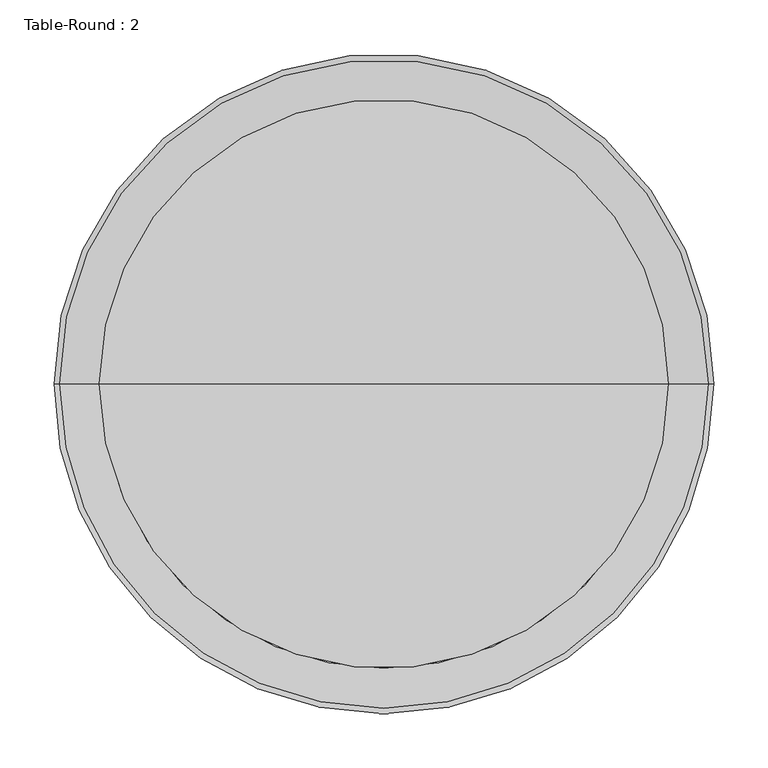
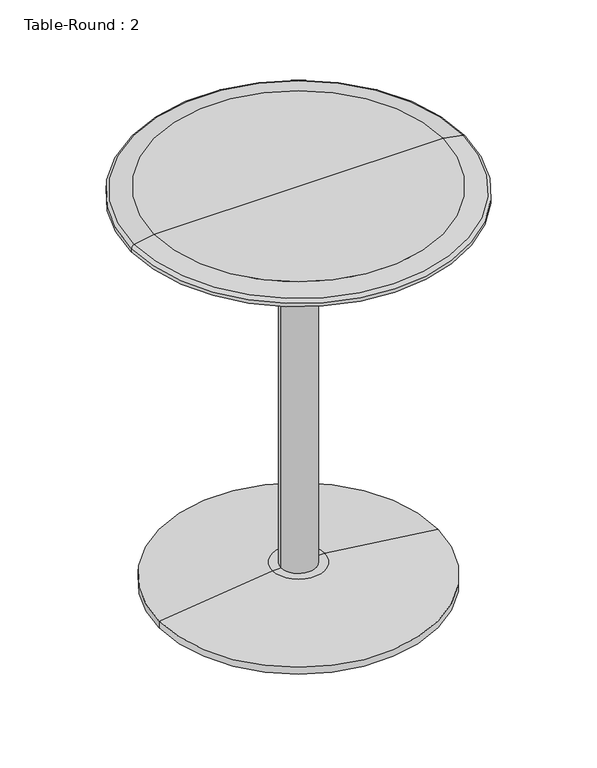
"""IFC4 building model written with IfcOpenShell, lengths in millimetres: furniture geometry, Table-Round : 2."""

from ifc_helpers import new_model, si_unit, point, frame, origin, origin_2d, place, context, project, spatial, polyline, circle_curve, ellipse_curve, trimmed, segment, composite_curve, outline, extrude, source, transform, mapped, element, save
from ifc_brep_helpers import plane_surface, cylinder_surface, revolved_surface, advanced_brep


def table_round_2_a0cc3393(model_context):
    return source(origin(), model_context, "Body", "SolidModel", [
        extrude(outline(composite_curve([segment(trimmed(circle_curve(origin_2d(), 31.75), [point((-31.75, 0.0))], [point((31.75, 0.0))], False, "CARTESIAN"), True, "CONTINUOUS"), segment(trimmed(circle_curve(origin_2d(), 31.75), [point((31.75, 0.0))], [point((-31.75, 0.0))], False, "CARTESIAN"), True, "CONTINUOUS")], self_intersect=False)), frame((0.0, 0.0, 38.1), z_axis=(0.0, 0.0, 1.0), x_axis=(1.0, 0.0, 0.0)), (0.0, 0.0, 1.0), 704.85),
        advanced_brep(
        [(0.0, 0.0, 742.95), (-304.8, 0.0, 742.95), (304.8, 0.0, 742.95), (262.9011364, 0.0, 762.0), (-262.9011364, 0.0, 762.0), (0.0, 0.0, 762.0), (299.5526659, 0.0, 755.5373465), (-299.5526659, 0.0, 755.5373465), (304.8, 0.0, 749.2838172), (-304.8, 0.0, 749.2838172)],
        [
            (0, 1),
            (1, 2, circle_curve(frame((0.0, 0.0, 742.95), z_axis=(0.0, 0.0, -1.0), x_axis=(-1.0, 0.0, 0.0)), 304.8)),
            (2, 0),
            (2, 1, circle_curve(frame((0.0, 0.0, 742.95), z_axis=(0.0, 0.0, -1.0), x_axis=(-1.0, 0.0, 0.0)), 304.8)),
            (3, 4, circle_curve(frame((0.0, 0.0, 762.0), z_axis=(0.0, 0.0, 1.0), x_axis=(-1.0, 0.0, 0.0)), 262.9011364)),
            (4, 5),
            (5, 3),
            (4, 3, circle_curve(frame((0.0, 0.0, 762.0), z_axis=(0.0, 0.0, 1.0), x_axis=(-1.0, 0.0, 0.0)), 262.9011364)),
            (6, 7, circle_curve(frame((0.0, 0.0, 755.5373465), z_axis=(0.0, 0.0, 1.0), x_axis=(-1.0, 0.0, 0.0)), 299.5526659)),
            (7, 4),
            (3, 6),
            (7, 6, circle_curve(frame((0.0, 0.0, 755.5373465), z_axis=(0.0, 0.0, 1.0), x_axis=(-1.0, 0.0, 0.0)), 299.5526659)),
            (8, 9, circle_curve(frame((0.0, 0.0, 749.2838172), z_axis=(0.0, 0.0, 1.0), x_axis=(-1.0, 0.0, 0.0)), 304.8)),
            (9, 7, circle_curve(frame((-298.45, 0.0, 749.2838172), z_axis=(0.0, 1.0, 0.0), x_axis=(1.0, 0.0, 0.0)), 6.35)),
            (6, 8, circle_curve(frame((298.45, 0.0, 749.2838172), z_axis=(0.0, 1.0, 0.0), x_axis=(-1.0, 0.0, 0.0)), 6.35)),
            (9, 8, circle_curve(frame((0.0, 0.0, 749.2838172), z_axis=(0.0, 0.0, 1.0), x_axis=(-1.0, 0.0, 0.0)), 304.8)),
            (1, 9),
            (8, 2),
        ],
        [
            plane_surface(frame((0.0, 0.0, 742.95), z_axis=(0.0, 0.0, -1.0), x_axis=(-1.0, 0.0, 0.0))),
            plane_surface(frame((0.0, 0.0, 762.0), z_axis=(0.0, 0.0, 1.0), x_axis=(-1.0, 0.0, 0.0))),
            revolved_surface(polyline([(-262.9011364, 0.0, 762.0), (-299.5526659, 0.0, 755.5373465)]), (0.0, 0.0, 838.2), (0.0, 0.0, -1.0)),
            revolved_surface(trimmed(ellipse_curve(frame((-298.45, 0.0, 749.2838172), z_axis=(0.0, -1.0, 0.0), x_axis=(1.0, 0.0, 0.0)), 6.35, 6.35), [point((-299.5526659, 0.0, 755.5373465))], [point((-304.8, 0.0, 749.2838172))], True, "CARTESIAN"), (0.0, 0.0, 838.2), (0.0, 0.0, -1.0)),
            cylinder_surface(frame((0.0, 0.0, 838.2), z_axis=(0.0, 0.0, -1.0), x_axis=(-1.0, 0.0, 0.0)), 304.8),
        ],
        [
            (0, [[1, 2, 3]]),
            (0, [[-3, 4, -1]]),
            (1, [[5, 6, 7]]),
            (1, [[8, -7, -6]]),
            (2, [[9, 10, -5, 11]]),
            (2, [[12, -11, -8, -10]]),
            (3, [[13, 14, -9, 15]]),
            (3, [[16, -15, -12, -14]]),
            (4, [[-2, 17, -13, 18]]),
            (4, [[-4, -18, -16, -17]]),
        ],
    ),
        advanced_brep(
        [(0.0, 0.0, 0.0), (-254.0, 0.0, 0.0), (254.0, 0.0, 0.0), (47.625, 0.0, 38.1), (-47.625, 0.0, 38.1), (0.0, 0.0, 38.1), (254.0, 0.0, 12.7), (-254.0, 0.0, 12.7)],
        [
            (0, 1),
            (1, 2, circle_curve(frame((0.0, 0.0, 0.0), z_axis=(0.0, 0.0, -1.0), x_axis=(-1.0, 0.0, 0.0)), 254.0)),
            (2, 0),
            (2, 1, circle_curve(frame((0.0, 0.0, 0.0), z_axis=(0.0, 0.0, -1.0), x_axis=(-1.0, 0.0, 0.0)), 254.0)),
            (3, 4, circle_curve(frame((0.0, 0.0, 38.1), z_axis=(0.0, 0.0, 1.0), x_axis=(-1.0, 0.0, 0.0)), 47.625)),
            (4, 5),
            (5, 3),
            (4, 3, circle_curve(frame((0.0, 0.0, 38.1), z_axis=(0.0, 0.0, 1.0), x_axis=(-1.0, 0.0, 0.0)), 47.625)),
            (6, 7, circle_curve(frame((0.0, 0.0, 12.7), z_axis=(0.0, 0.0, 1.0), x_axis=(-1.0, 0.0, 0.0)), 254.0)),
            (7, 4),
            (3, 6),
            (7, 6, circle_curve(frame((0.0, 0.0, 12.7), z_axis=(0.0, 0.0, 1.0), x_axis=(-1.0, 0.0, 0.0)), 254.0)),
            (1, 7),
            (6, 2),
        ],
        [
            plane_surface(frame((0.0, 0.0, 0.0), z_axis=(0.0, 0.0, -1.0), x_axis=(-1.0, 0.0, 0.0))),
            plane_surface(frame((0.0, 0.0, 38.1), z_axis=(0.0, 0.0, 1.0), x_axis=(-1.0, 0.0, 0.0))),
            revolved_surface(polyline([(-47.625, 0.0, 38.1), (-254.0, 0.0, 12.7)]), (0.0, 0.0, 215.9), (0.0, 0.0, -1.0)),
            cylinder_surface(frame((0.0, 0.0, 215.9), z_axis=(0.0, 0.0, -1.0), x_axis=(-1.0, 0.0, 0.0)), 254.0),
        ],
        [
            (0, [[1, 2, 3]]),
            (0, [[-3, 4, -1]]),
            (1, [[5, 6, 7]]),
            (1, [[8, -7, -6]]),
            (2, [[9, 10, -5, 11]]),
            (2, [[12, -11, -8, -10]]),
            (3, [[-2, 13, -9, 14]]),
            (3, [[-4, -14, -12, -13]]),
        ],
    ),
    ])


if __name__ == "__main__":
    model = new_model("IFC4")
    model_context = context("Model", 3, world=origin())
    ifc_project = project(units=[si_unit("LENGTHUNIT", "METRE", prefix="MILLI")], contexts=[model_context])
    site = spatial("IfcSite", under=ifc_project)
    building = spatial("IfcBuilding", under=site)
    placement = place(None, origin())
    table_round_2_shape = table_round_2_a0cc3393(model_context)
    element("IfcFurniture", 1, ObjectType="Table-Round : 2", at=placement, inside=building, context=model_context, shape_type="MappedRepresentation", body=[
        mapped(table_round_2_shape, transform((0.0, 0.0, 0.0), x_axis=(1.0, 0.0, 0.0), y_axis=(0.0, 1.0, 0.0), z_axis=(0.0, 0.0, 1.0))),
    ])
    save(model, "model.ifc")

# Revit data of these elements
# Type "Table-Round : 2"
#   Assembly Code = "E2020200"
#   Base Radius = 0' - 10"
#   Height = 2' - 6"
#   Radius = 1' - 0"
#   Base Material = Steel, Chrome Plated
#   Top Material = Birch
#   Default Elevation = 0
# Element 1 (IfcFurniture, "Table-Round : 2")
#   Materials on its faces: "Steel, Chrome Plated", "Birch"
# Materials
#   "Steel, Chrome Plated": class "Metal", colour RGB 17 17 17, transparency 0, Description = "Chromiuim plated steel", Cost = 0
#   "Birch": class "Wood", colour RGB 224 178 126, transparency 0, Description = "Betula Alleghaniensis", Cost = 0
